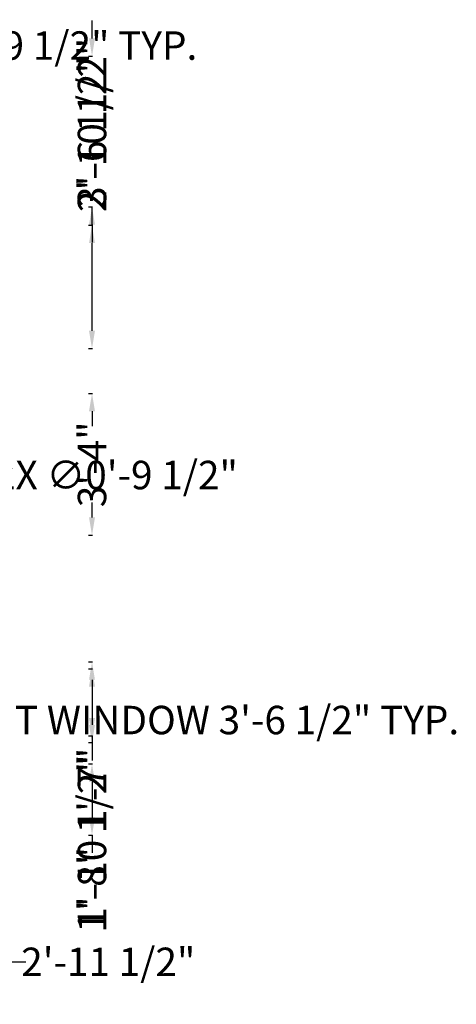
# Model space of a CAD drawing. Units: inches. Extents: x -52 to 493, y -432 to 100.
# Tile 4 of 5: x 370 to 493, y -432 to -155. Entities that reach past the tile are written whole.
import ezdxf

# ---------------------------------------------------------------- set-up
doc = ezdxf.new("R2010")
doc.units = ezdxf.units.IN
doc.header["$MEASUREMENT"] = 0
doc.layers.add('A-ANNO-DIMS', color=2, linetype='Continuous', lineweight=18)
doc.styles.get("Standard").update_dxf_attribs({"font": 'arial.ttf'})
doc.dimstyles.get("Standard").update_dxf_attribs({"dimtxt": 8, "dimasz": 5, "dimexe": 0.18, "dimexo": 0.0625, "dimgap": 0.09, "dimtad": 0, "dimdec": 0, "dimzin": 0, "dimdsep": 46, "dimlunit": 3, "dimtxsty": 'Standard', "dimcen": 0.09, "dimadec": 0, "dimazin": 0, "dimtfac": 1, "dimtdec": 0, "dimtofl": 0, "dimtmove": 0, "dimatfit": 3, "dimfxl": 1, "dimfxlon": 1, "dimtolj": 1, "dimtzin": 0, "dimarcsym": 0})

# ---------------------------------------------------------------- blocks, each defined once
blk = doc.blocks.new('*D36')
at = {"layer": 'A-ANNO-DIMS', "color": 0, "lineweight": -2, "transparency": 16777216}
for p, q in [((288.89, -353.27), (288.89, -352.09)), ((293.89, -352.27), (326.2, -352.27)), ((331.2, -353.27), (331.2, -352.09)), ((331.2, -352.27), (336.2, -352.27))]:
    blk.add_line(p, q, dxfattribs=at)
at = {"layer": 'A-ANNO-DIMS', "color": 0, "transparency": 16777216}
for points in [[(293.89, -351.44), (293.89, -353.1), (288.89, -352.27)], [(326.2, -351.44), (326.2, -353.1), (331.2, -352.27)]]:
    blk.add_solid(points, dxfattribs=at)
at = {"layer": 'Defpoints', "color": 0, "transparency": 16777216}
for p in [(331.2, -352.27), (288.89, -358.62), (331.2, -358.62)]:
    blk.add_point(p, dxfattribs=at)
at = {"layer": 'A-ANNO-DIMS', "color": 0, "transparency": 16777216, "insert": (416.63, -352.27), "char_height": 8, "attachment_point": 5}
blk.add_mtext('\\A1;FRONT WINDOW 3\'-6 1/2" TYP.', dxfattribs=at)
blk = doc.blocks.new('*D44')
at = {"layer": 'A-ANNO-DIMS', "color": 0, "lineweight": -2, "transparency": 16777216}
for p, q in [((349.88, -208.05), (351.06, -208.05)), ((350.88, -213.05), (350.88, -216.46)), ((349.88, -221.46), (351.06, -221.46)), ((350.88, -221.46), (350.88, -226.46))]:
    blk.add_line(p, q, dxfattribs=at)
at = {"layer": 'A-ANNO-DIMS', "color": 0, "transparency": 16777216}
for points in [[(350.04, -213.05), (351.71, -213.05), (350.88, -208.05)], [(350.04, -216.46), (351.71, -216.46), (350.88, -221.46)]]:
    blk.add_solid(points, dxfattribs=at)
at = {"layer": 'Defpoints', "color": 0, "transparency": 16777216}
for p in [(348.87, -208.05), (348.87, -221.46), (350.88, -221.46)]:
    blk.add_point(p, dxfattribs=at)
at = {"layer": 'A-ANNO-DIMS', "color": 0, "transparency": 16777216, "insert": (350.88, -300.1), "char_height": 8, "attachment_point": 5, "rotation": 90}
blk.add_mtext('\\A1;DINING CHAIR 1\'-1 1/2" TYP.', dxfattribs=at)
blk = doc.blocks.new('*D46')
at = {"layer": 'A-ANNO-DIMS', "color": 0, "lineweight": -2, "transparency": 16777216}
for p, q in [((246.2, -161.73), (246.2, -162.91)), ((251.2, -162.73), (310.69, -162.73)), ((315.69, -161.73), (315.69, -162.91)), ((315.69, -162.73), (320.69, -162.73))]:
    blk.add_line(p, q, dxfattribs=at)
at = {"layer": 'A-ANNO-DIMS', "color": 0, "transparency": 16777216}
for points in [[(251.2, -161.9), (251.2, -163.56), (246.2, -162.73)], [(310.69, -161.9), (310.69, -163.56), (315.69, -162.73)]]:
    blk.add_solid(points, dxfattribs=at)
at = {"layer": 'Defpoints', "color": 0, "transparency": 16777216}
for p in [(246.2, -152.31), (315.69, -152.31), (315.69, -162.73)]:
    blk.add_point(p, dxfattribs=at)
at = {"layer": 'A-ANNO-DIMS', "color": 0, "transparency": 16777216, "insert": (371.23, -162.73), "char_height": 8, "attachment_point": 5}
blk.add_mtext('\\A1;SOFA 5\'-9 1/2" TYP.', dxfattribs=at)
blk = doc.blocks.new('*D62')
at = {"layer": 'A-ANNO-DIMS', "color": 0, "lineweight": -2, "transparency": 16777216}
for p, q in [((390.3, -213.25), (390.3, -208.25)), ((389.3, -213.25), (390.48, -213.25)), ((390.3, -242.89), (390.3, -218.25)), ((389.3, -247.89), (390.48, -247.89))]:
    blk.add_line(p, q, dxfattribs=at)
at = {"layer": 'A-ANNO-DIMS', "color": 0, "transparency": 16777216}
for points in [[(389.46, -218.25), (391.13, -218.25), (390.3, -213.25)], [(389.46, -242.89), (391.13, -242.89), (390.3, -247.89)]]:
    blk.add_solid(points, dxfattribs=at)
at = {"layer": 'Defpoints', "color": 0, "transparency": 16777216}
for p in [(366.65, -213.25), (390.3, -213.25), (366.65, -247.89)]:
    blk.add_point(p, dxfattribs=at)
at = {"layer": 'A-ANNO-DIMS', "color": 0, "transparency": 16777216, "insert": (390.3, -185.03), "char_height": 8, "attachment_point": 5, "rotation": 90}
blk.add_mtext('\\A1;2\'-10 1/2"', dxfattribs=at)
blk = doc.blocks.new('*D65')
at = {"layer": 'A-ANNO-DIMS', "color": 0, "lineweight": -2, "transparency": 16777216}
for p, q in [((331.2, -419.22), (331.2, -420.4)), ((336.2, -420.22), (361.65, -420.22)), ((366.65, -419.22), (366.65, -420.4)), ((366.65, -420.22), (371.65, -420.22))]:
    blk.add_line(p, q, dxfattribs=at)
at = {"layer": 'A-ANNO-DIMS', "color": 0, "transparency": 16777216}
for points in [[(336.2, -419.39), (336.2, -421.06), (331.2, -420.22)], [(361.65, -419.39), (361.65, -421.06), (366.65, -420.22)]]:
    blk.add_solid(points, dxfattribs=at)
at = {"layer": 'Defpoints', "color": 0, "transparency": 16777216}
for p in [(331.2, -364.62), (366.65, -364.62), (366.65, -420.22)]:
    blk.add_point(p, dxfattribs=at)
at = {"layer": 'A-ANNO-DIMS', "color": 0, "transparency": 16777216, "insert": (394.87, -420.22), "char_height": 8, "attachment_point": 5}
blk.add_mtext('\\A1;2\'-11 1/2"', dxfattribs=at)
blk = doc.blocks.new('*D66')
at = {"layer": 'A-ANNO-DIMS', "color": 0, "lineweight": -2, "transparency": 16777216}
for p, q in [((389.3, -364.62), (390.48, -364.62)), ((390.3, -369.62), (390.3, -379.62)), ((389.3, -384.62), (390.48, -384.62)), ((390.3, -384.62), (390.3, -389.62))]:
    blk.add_line(p, q, dxfattribs=at)
at = {"layer": 'A-ANNO-DIMS', "color": 0, "transparency": 16777216}
for points in [[(389.46, -369.62), (391.13, -369.62), (390.3, -364.62)], [(389.46, -379.62), (391.13, -379.62), (390.3, -384.62)]]:
    blk.add_solid(points, dxfattribs=at)
at = {"layer": 'Defpoints', "color": 0, "transparency": 16777216}
for p in [(255.65, -364.62), (255.65, -384.62), (390.3, -384.62)]:
    blk.add_point(p, dxfattribs=at)
at = {"layer": 'A-ANNO-DIMS', "color": 0, "transparency": 16777216, "insert": (390.3, -399.96), "char_height": 8, "attachment_point": 5, "rotation": 90}
blk.add_mtext('\\A1;1\'-8"', dxfattribs=at)
blk = doc.blocks.new('*D73')
at = {"layer": 'A-ANNO-DIMS', "color": 0, "lineweight": -2, "transparency": 16777216}
for p, q in [((389.3, -260.49), (390.48, -260.49)), ((390.3, -265.49), (390.3, -269.69)), ((390.3, -295.34), (390.3, -291.13)), ((389.3, -300.34), (390.48, -300.34))]:
    blk.add_line(p, q, dxfattribs=at)
at = {"layer": 'A-ANNO-DIMS', "color": 0, "transparency": 16777216}
for points in [[(389.46, -265.49), (391.13, -265.49), (390.3, -260.49)], [(389.46, -295.34), (391.13, -295.34), (390.3, -300.34)]]:
    blk.add_solid(points, dxfattribs=at)
at = {"layer": 'Defpoints', "color": 0, "transparency": 16777216}
for p in [(261.65, -260.49), (261.65, -300.34), (390.3, -300.34)]:
    blk.add_point(p, dxfattribs=at)
at = {"layer": 'A-ANNO-DIMS', "color": 0, "transparency": 16777216, "insert": (390.3, -280.41), "char_height": 8, "attachment_point": 5, "rotation": 90}
blk.add_mtext('\\A1;3\'-4"', dxfattribs=at)
blk = doc.blocks.new('*D74')
at = {"layer": 'A-ANNO-DIMS', "color": 0, "lineweight": -2, "transparency": 16777216}
for p, q in [((334.72, 87.29), (334.72, 88.47)), ((339.72, 88.29), (352.65, 88.29)), ((357.65, 87.29), (357.65, 88.47)), ((357.65, 88.29), (362.65, 88.29))]:
    blk.add_line(p, q, dxfattribs=at)
at = {"layer": 'A-ANNO-DIMS', "color": 0, "transparency": 16777216}
for points in [[(339.72, 89.13), (339.72, 87.46), (334.72, 88.29)], [(352.65, 89.13), (352.65, 87.46), (357.65, 88.29)]]:
    blk.add_solid(points, dxfattribs=at)
at = {"layer": 'Defpoints', "color": 0, "transparency": 16777216}
for p in [(357.65, 88.29), (334.72, -335.93), (357.65, -358.62)]:
    blk.add_point(p, dxfattribs=at)
at = {"layer": 'A-ANNO-DIMS', "color": 0, "transparency": 16777216, "insert": (376.1, 88.29), "char_height": 8, "attachment_point": 5}
blk.add_mtext('\\A1;1\'-11"', dxfattribs=at)
blk = doc.blocks.new('*D75')
at = {"layer": 'A-ANNO-DIMS', "color": 0, "lineweight": -2, "transparency": 16777216}
for p, q in [((389.3, -335.93), (390.48, -335.93)), ((390.3, -340.93), (390.3, -353.62)), ((389.3, -358.62), (390.48, -358.62)), ((390.3, -358.62), (390.3, -363.62))]:
    blk.add_line(p, q, dxfattribs=at)
at = {"layer": 'A-ANNO-DIMS', "color": 0, "transparency": 16777216}
for points in [[(389.46, -340.93), (391.13, -340.93), (390.3, -335.93)], [(389.46, -353.62), (391.13, -353.62), (390.3, -358.62)]]:
    blk.add_solid(points, dxfattribs=at)
at = {"layer": 'Defpoints', "color": 0, "transparency": 16777216}
for p in [(334.72, -335.93), (331.2, -358.62), (390.3, -358.62)]:
    blk.add_point(p, dxfattribs=at)
at = {"layer": 'A-ANNO-DIMS', "color": 0, "transparency": 16777216, "insert": (390.3, -386.39), "char_height": 8, "attachment_point": 5, "rotation": 90}
blk.add_mtext('\\A1;1\'-10 1/2"', dxfattribs=at)
blk = doc.blocks.new('*D77')
at = {"layer": 'A-ANNO-DIMS', "color": 0, "lineweight": -2, "transparency": 16777216}
for p, q in [((390.3, -160.71), (390.3, -155.71)), ((389.3, -165.71), (390.48, -165.71)), ((389.3, -208.05), (390.48, -208.05)), ((390.3, -213.05), (390.3, -218.05))]:
    blk.add_line(p, q, dxfattribs=at)
at = {"layer": 'A-ANNO-DIMS', "color": 0, "transparency": 16777216}
for points in [[(389.46, -160.71), (391.13, -160.71), (390.3, -165.71)], [(389.46, -213.05), (391.13, -213.05), (390.3, -208.05)]]:
    blk.add_solid(points, dxfattribs=at)
at = {"layer": 'Defpoints', "color": 0, "transparency": 16777216}
for p in [(354.16, -165.71), (354.16, -208.05), (390.3, -208.05)]:
    blk.add_point(p, dxfattribs=at)
at = {"layer": 'A-ANNO-DIMS', "color": 0, "transparency": 16777216, "insert": (390.3, -186.88), "char_height": 8, "attachment_point": 5, "rotation": 90}
blk.add_mtext('\\A1;3\'-6 1/2"', dxfattribs=at)
blk = doc.blocks.new('*D83')
at = {"layer": 'A-ANNO-DIMS', "color": 0, "lineweight": -2, "transparency": 16777216}
for p, q in [((389.3, -337.87), (390.48, -337.87)), ((390.3, -342.87), (390.3, -351.72)), ((389.3, -356.72), (390.48, -356.72)), ((390.3, -356.72), (390.3, -361.72))]:
    blk.add_line(p, q, dxfattribs=at)
at = {"layer": 'A-ANNO-DIMS', "color": 0, "transparency": 16777216}
for points in [[(389.46, -342.87), (391.13, -342.87), (390.3, -337.87)], [(389.46, -351.72), (391.13, -351.72), (390.3, -356.72)]]:
    blk.add_solid(points, dxfattribs=at)
at = {"layer": 'Defpoints', "color": 0, "transparency": 16777216}
for p in [(280.41, -337.87), (280.41, -356.72), (390.3, -356.72)]:
    blk.add_point(p, dxfattribs=at)
at = {"layer": 'A-ANNO-DIMS', "color": 0, "transparency": 16777216, "insert": (390.3, -372.07), "char_height": 8, "attachment_point": 5, "rotation": 90}
blk.add_mtext('\\A1;1\'-7"', dxfattribs=at)
blk = doc.blocks.new('*D84')
at = {"layer": 'A-ANNO-DIMS', "color": 0, "lineweight": -2, "transparency": 16777216}
for p, q in [((349.33, -283.41), (349.51, -283.41)), ((349.42, -283.5), (349.42, -283.32)), ((364.19, -283.41), (359.19, -283.41))]:
    blk.add_line(p, q, dxfattribs=at)
at = {"layer": 'A-ANNO-DIMS', "color": 0, "transparency": 16777216}
blk.add_solid([(359.19, -282.58), (359.19, -284.25), (354.19, -283.41)], dxfattribs=at)
at = {"layer": 'Defpoints', "color": 0, "transparency": 16777216}
for p in [(344.65, -283.41), (354.19, -283.41)]:
    blk.add_point(p, dxfattribs=at)
at = {"layer": 'A-ANNO-DIMS', "color": 0, "transparency": 16777216, "insert": (397.03, -283.42), "char_height": 8, "attachment_point": 5, "rotation": 359.9944}
blk.add_mtext('\\A1;2X ∅0\'-9 1/2"', dxfattribs=at)

msp = doc.modelspace()

# ---------------------------------------------------------------- dimensions: what is measured, and where the dimension line sits
at = {"layer": 'A-ANNO-DIMS'}
for base, p1, p2, picture, middle in [((357.65, 88.29), (334.72, -335.93), (357.65, -358.62), '*D74', (376.1, 88.29)), ((366.6476, -420.2223), (331.1965, -364.616), (366.6476, -364.616), '*D65', (394.8672, -420.2223))]:
    dim = msp.add_linear_dim(base=base, p1=p1, p2=p2, dimstyle='Standard', override={"dimdec": 1, "dimlfac": 1, "dimrnd": 0, "dimzin": 1, "dimdsep": 46, "dimlunit": 4, "dimfrac": 2}, dxfattribs=at)
    dim.commit()
    dim.dimension.update_dxf_attribs({"geometry": picture, "text_midpoint": middle})
for base, p1, p2, text, picture, middle in [((315.69, -162.73), (246.2, -152.31), (315.69, -152.31), 'SOFA <> TYP.', '*D46', (371.23, -162.73)), ((331.2, -352.27), (288.89, -358.62), (331.2, -358.62), 'FRONT WINDOW <> TYP.', '*D36', (416.63, -352.27))]:
    dim = msp.add_linear_dim(base=base, p1=p1, p2=p2, text=text, dimstyle='Standard', override={"dimdec": 1, "dimlfac": 1, "dimrnd": 0, "dimzin": 1, "dimdsep": 46, "dimlunit": 4, "dimfrac": 2}, dxfattribs=at)
    dim.commit()
    dim.dimension.update_dxf_attribs({"geometry": picture, "text_midpoint": middle})
for base, p1, p2, picture, middle in [((390.3, -208.05), (354.16, -165.71), (354.16, -208.05), '*D77', (390.3, -186.88)), ((390.3, -213.25), (366.65, -247.89), (366.65, -213.25), '*D62', (390.3, -185.03)), ((390.2976, -300.3373), (261.6476, -260.4891), (261.6476, -300.3373), '*D73', (390.2976, -280.4132)), ((390.3, -358.62), (334.72, -335.93), (331.2, -358.62), '*D75', (390.3, -386.39)), ((390.2976, -356.7247), (280.409, -337.871), (280.409, -356.7247), '*D83', (390.2976, -372.0711)), ((390.3, -384.62), (255.65, -364.62), (255.65, -384.62), '*D66', (390.3, -399.96))]:
    dim = msp.add_linear_dim(base=base, p1=p1, p2=p2, angle=90, dimstyle='Standard', override={"dimdec": 1, "dimlfac": 1, "dimrnd": 0, "dimzin": 1, "dimdsep": 46, "dimlunit": 4, "dimfrac": 2}, dxfattribs=at)
    dim.commit()
    dim.dimension.update_dxf_attribs({"geometry": picture, "text_midpoint": middle})
dim = msp.add_linear_dim(base=(350.88, -221.46), p1=(348.87, -208.05), p2=(348.87, -221.46), angle=270, text='DINING CHAIR <> TYP.', dimstyle='Standard', override={"dimdec": 1, "dimlfac": 1, "dimrnd": 0, "dimzin": 1, "dimdsep": 46, "dimlunit": 4, "dimfrac": 2}, dxfattribs=at)
dim.commit()
dim.dimension.update_dxf_attribs({"geometry": '*D44', "text_midpoint": (350.88, -300.1)})
dim = msp.add_diameter_dim_2p(p1=(344.65, -283.41), p2=(354.19, -283.41), text='2X <>', dimstyle='Standard', override={"dimdec": 1, "dimlfac": 1, "dimrnd": 0, "dimzin": 1, "dimdsep": 46, "dimlunit": 4, "dimfrac": 2}, dxfattribs=at)
dim.commit()
dim.dimension.update_dxf_attribs({"geometry": '*D84', "text_midpoint": (397.03, -283.42)})

doc.saveas('drawing.dxf')
